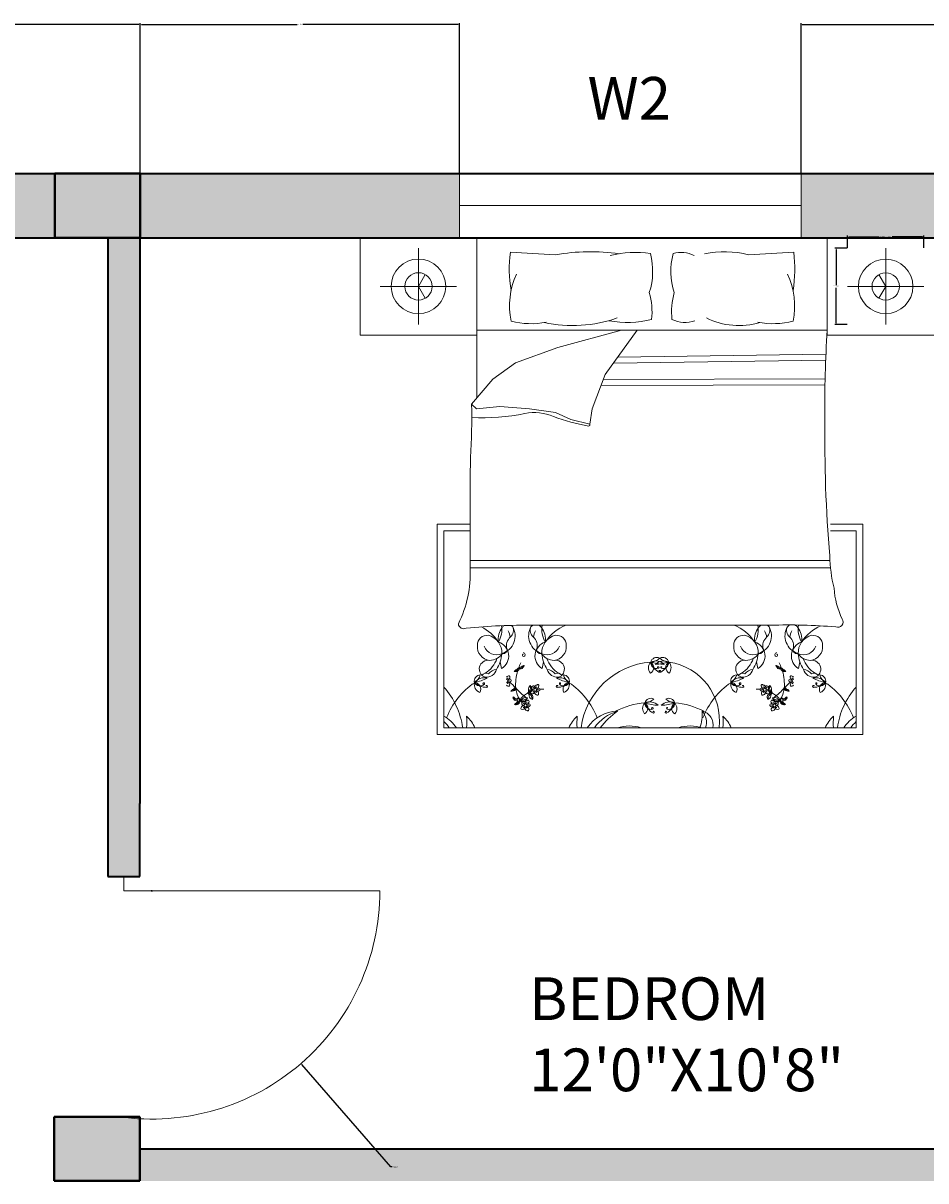
# Model space of a CAD drawing. Units: inches. Extents: x 1623 to 2200, y 2019 to 3010.
# Tile 4 of 6: x 1902 to 2029, y 2342 to 2505. Entities that reach past the tile are written whole.
import ezdxf

# ---------------------------------------------------------------- set-up
doc = ezdxf.new("R2010")
doc.units = ezdxf.units.IN
for name, color, linetype, lineweight in [('A-ANNO-DIMS', 2, 'Continuous', 18), ('A-AREA-IDEN', 7, 'Continuous', 18), ('A-COLS', 7, 'Continuous', 40), ('A-DOOR', 3, 'Continuous', 18), ('A-FURN', 8, 'Continuous', 13), ('A-GLAZ', 4, 'Continuous', 18), ('A-GLAZ-IDEN', 7, 'Continuous', 18), ('A-WALL', 7, 'Continuous', 35)]:
    doc.layers.add(name, color=color, linetype=linetype, lineweight=lineweight)
doc.layers.add('A-COLS-PATT', color=152, linetype='Continuous', lineweight=13, true_color=0x2776bb)
doc.layers.add('A-WALL-PATT', color=251, linetype='Continuous', lineweight=13, true_color=0x636466)
doc.styles.get("Standard").update_dxf_attribs({"font": 'arial.ttf'})
doc.dimstyles.get("Standard").update_dxf_attribs({"dimtxt": 0.18, "dimasz": 0.18, "dimexe": 0.18, "dimexo": 0.0625, "dimgap": 0.09, "dimtad": 0, "dimtih": 1, "dimtoh": 1, "dimdec": 4, "dimzin": 0, "dimdsep": 46, "dimtxsty": 'Standard', "dimcen": 0.09, "dimadec": 0, "dimazin": 0, "dimtfac": 1, "dimtdec": 4, "dimtofl": 0, "dimtmove": 0, "dimatfit": 3, "dimfxl": 1, "dimtolj": 1, "dimtzin": 0, "dimarcsym": 0})

# ---------------------------------------------------------------- blocks, each defined once
blk = doc.blocks.new('COL-12X9-PLAN')
for p, q in [((0, 0), (0, 9)), ((0, 9), (12, 9)), ((12, 9), (12, 0)), ((9, 0), (0, 0)), ((12, 0), (9, 0))]:
    blk.add_line(p, q)
blk = doc.blocks.new('WIN-48-PLAN')
for p, q in [((0, 9), (0, 0)), ((48, 4.5), (48, 9)), ((48, 9), (48, 0)), ((0, 0), (0, 4.5)), ((0, 4.5), (48, 4.5))]:
    blk.add_line(p, q)
blk = doc.blocks.new('BEDSIDE-LAMP-PLAN')
for p, q in [((5.36, 0), (5.36, 10.73)), ((0, 5.36), (10.73, 5.36))]:
    blk.add_line(p, q)
for points in [[(5.36, 5.36), (4.41, 7.02)], [(5.36, 5.36), (4.41, 3.7)]]:
    blk.add_lwpolyline(points)
for radius in [3.83, 1.92]:
    blk.add_circle((5.36, 5.36), radius)
blk = doc.blocks.new('*D16')
at = {"layer": 'A-ANNO-DIMS', "color": 0, "lineweight": -2, "transparency": 16777216}
for p, q in [((2017.8, 2473.11), (2017.8, 2474.84)), ((2017.98, 2474.66), (2022.26, 2474.66)), ((2028.34, 2474.66), (2024.06, 2474.66)), ((2028.52, 2473.11), (2028.52, 2474.84))]:
    blk.add_line(p, q, dxfattribs=at)
at = {"layer": 'A-ANNO-DIMS', "color": 0, "transparency": 16777216}
for points in [[(2017.98, 2474.69), (2017.98, 2474.63), (2017.8, 2474.66)], [(2028.34, 2474.69), (2028.34, 2474.63), (2028.52, 2474.66)]]:
    blk.add_solid(points, dxfattribs=at)
at = {"layer": 'Defpoints', "color": 0, "transparency": 16777216}
for p in [(2028.52, 2474.66), (2017.8, 2473.05), (2028.52, 2473.05)]:
    blk.add_point(p, dxfattribs=at)
at = {"layer": 'A-ANNO-DIMS', "color": 0, "transparency": 16777216, "insert": (2023.16, 2474.66), "char_height": 0.18, "attachment_point": 5}
blk.add_mtext('\\A1;LAMP 11 TYP.', dxfattribs=at)
blk = doc.blocks.new('*D17')
at = {"layer": 'A-ANNO-DIMS', "color": 0, "lineweight": -2, "transparency": 16777216}
for p, q in [((2017.73, 2473.05), (2016.01, 2473.05)), ((2016.19, 2472.87), (2016.19, 2467.86)), ((2016.19, 2462.5), (2016.19, 2467.5)), ((2017.73, 2462.32), (2016.01, 2462.32))]:
    blk.add_line(p, q, dxfattribs=at)
at = {"layer": 'A-ANNO-DIMS', "color": 0, "transparency": 16777216}
for points in [[(2016.16, 2472.87), (2016.22, 2472.87), (2016.19, 2473.05)], [(2016.16, 2462.5), (2016.22, 2462.5), (2016.19, 2462.32)]]:
    blk.add_solid(points, dxfattribs=at)
at = {"layer": 'Defpoints', "color": 0, "transparency": 16777216}
for p in [(2016.19, 2473.05), (2017.8, 2473.05), (2017.8, 2462.32)]:
    blk.add_point(p, dxfattribs=at)
at = {"layer": 'A-ANNO-DIMS', "color": 0, "transparency": 16777216, "insert": (2016.19, 2467.68), "char_height": 0.18, "attachment_point": 5}
blk.add_mtext('\\A1;11 TYP.', dxfattribs=at)
blk = doc.blocks.new('*D34')
at = {"layer": 'A-ANNO-DIMS', "color": 0, "lineweight": -2, "transparency": 16777216}
for p, q in [((1878.5, 2483.59), (1878.5, 2504.66)), ((1918.4, 2483.59), (1918.4, 2504.66)), ((1878.68, 2504.48), (1898.12, 2504.48)), ((1918.22, 2504.48), (1898.77, 2504.48))]:
    blk.add_line(p, q, dxfattribs=at)
at = {"layer": 'A-ANNO-DIMS', "color": 0, "transparency": 16777216}
for points in [[(1878.68, 2504.51), (1878.68, 2504.45), (1878.5, 2504.48)], [(1918.22, 2504.51), (1918.22, 2504.45), (1918.4, 2504.48)]]:
    blk.add_solid(points, dxfattribs=at)
at = {"layer": 'Defpoints', "color": 0, "transparency": 16777216}
for p in [(1918.4, 2504.48), (1878.5, 2483.52), (1918.4, 2483.52)]:
    blk.add_point(p, dxfattribs=at)
at = {"layer": 'A-ANNO-DIMS', "color": 0, "transparency": 16777216, "insert": (1898.45, 2504.48), "char_height": 0.18, "attachment_point": 5}
blk.add_mtext('\\A1;39.9', dxfattribs=at)
blk = doc.blocks.new('*D35')
at = {"layer": 'A-ANNO-DIMS', "color": 0, "lineweight": -2, "transparency": 16777216}
for p, q in [((1918.4, 2483.59), (1918.4, 2504.66)), ((1963.26, 2483.59), (1963.26, 2504.66)), ((1918.58, 2504.48), (1940.43, 2504.48)), ((1963.08, 2504.48), (1941.23, 2504.48))]:
    blk.add_line(p, q, dxfattribs=at)
at = {"layer": 'A-ANNO-DIMS', "color": 0, "transparency": 16777216}
for points in [[(1918.58, 2504.51), (1918.58, 2504.45), (1918.4, 2504.48)], [(1963.08, 2504.51), (1963.08, 2504.45), (1963.26, 2504.48)]]:
    blk.add_solid(points, dxfattribs=at)
at = {"layer": 'Defpoints', "color": 0, "transparency": 16777216}
for p in [(1963.26, 2504.48), (1918.4, 2483.52), (1963.26, 2483.52)]:
    blk.add_point(p, dxfattribs=at)
at = {"layer": 'A-ANNO-DIMS', "color": 0, "transparency": 16777216, "insert": (1940.83, 2504.48), "char_height": 0.18, "attachment_point": 5}
blk.add_mtext('\\A1;44.86', dxfattribs=at)
blk = doc.blocks.new('*D36')
at = {"layer": 'A-ANNO-DIMS', "color": 0, "lineweight": -2, "transparency": 16777216}
for p, q in [((2011.26, 2483.59), (2011.26, 2504.66)), ((2071.33, 2483.59), (2071.33, 2504.66)), ((2011.44, 2504.48), (2040.9, 2504.48)), ((2071.15, 2504.48), (2041.69, 2504.48))]:
    blk.add_line(p, q, dxfattribs=at)
at = {"layer": 'A-ANNO-DIMS', "color": 0, "transparency": 16777216}
for points in [[(2011.44, 2504.51), (2011.44, 2504.45), (2011.26, 2504.48)], [(2071.15, 2504.51), (2071.15, 2504.45), (2071.33, 2504.48)]]:
    blk.add_solid(points, dxfattribs=at)
at = {"layer": 'Defpoints', "color": 0, "transparency": 16777216}
for p in [(2071.33, 2504.48), (2011.26, 2483.52), (2071.33, 2483.53)]:
    blk.add_point(p, dxfattribs=at)
at = {"layer": 'A-ANNO-DIMS', "color": 0, "transparency": 16777216, "insert": (2041.29, 2504.48), "char_height": 0.18, "attachment_point": 5}
blk.add_mtext('\\A1;60.07', dxfattribs=at)
blk = doc.blocks.new('*D63')
at = {"layer": 'A-ANNO-DIMS', "color": 0, "lineweight": -2, "transparency": 16777216}
for p, q in [((1919.92, 2382.76), (1920.1, 2382.76)), ((1920.01, 2382.67), (1920.01, 2382.85)), ((1953.6, 2343.98), (1941.12, 2358.39)), ((1953.78, 2343.98), (1953.6, 2343.98))]:
    blk.add_line(p, q, dxfattribs=at)
at = {"layer": 'A-ANNO-DIMS', "color": 0, "transparency": 16777216}
blk.add_solid([(1941.15, 2358.41), (1941.1, 2358.37), (1941.01, 2358.53)], dxfattribs=at)
at = {"layer": 'Defpoints', "color": 0, "transparency": 16777216}
for p in [(1920.01, 2382.76), (1941.01, 2358.53)]:
    blk.add_point(p, dxfattribs=at)
at = {"layer": 'A-ANNO-DIMS', "color": 0, "transparency": 16777216, "insert": (1954.26, 2343.98), "char_height": 0.18, "attachment_point": 5}
blk.add_mtext('\\A1;R32.06', dxfattribs=at)

msp = doc.modelspace()

# ---------------------------------------------------------------- hatches: boundary and pattern name
at = {"layer": 'A-COLS-PATT'}
h = msp.add_hatch(color=256, dxfattribs=at)
h.dxf.hatch_style = 1
h.paths.add_polyline_path([(1722.3258, 2483.5237), (1710.3258, 2483.5237), (1710.3258, 2474.5237), (1719.3258, 2474.5237), (1722.3258, 2474.5237)])
h.paths.add_polyline_path([(1809.3258, 2483.5237), (1797.3258, 2483.5237), (1797.3258, 2474.5237), (1806.3258, 2474.5237), (1809.3258, 2474.5237)])
h.paths.add_polyline_path([(1918.3972, 2483.5237), (1906.3972, 2483.5237), (1906.3972, 2474.5237), (1915.3972, 2474.5237), (1918.3972, 2474.5237)])
h.paths.add_polyline_path([(2071.3258, 2483.5237), (2059.3258, 2483.5237), (2059.3258, 2474.532), (2068.3258, 2474.532), (2071.3258, 2474.532)])
h.paths.add_polyline_path([(2071.3258, 2351.0312), (2059.3258, 2351.0312), (2059.3258, 2342.0312), (2068.3258, 2342.0312), (2071.3258, 2342.0312)])
h.paths.add_polyline_path([(1918.3258, 2351.0237), (1906.3258, 2351.0237), (1906.3258, 2342.0237), (1915.3258, 2342.0237), (1918.3258, 2342.0237)])
h.paths.add_polyline_path([(1722.3198, 2351.0237), (1710.3258, 2351.0237), (1710.3258, 2342.0237), (1719.3198, 2342.0237), (1722.3198, 2342.0237)])
h.paths.add_polyline_path([(1809.3158, 2351.0237), (1797.3258, 2351.0237), (1797.3258, 2346.5237), (1797.3158, 2342.0237), (1806.3158, 2342.0237), (1809.3158, 2342.0237)])
h.paths.add_polyline_path([(1722.3029, 2170.0237), (1710.3258, 2170.0237), (1710.3258, 2161.0237), (1714.3029, 2161.0237), (1719.3029, 2161.0237), (1722.3029, 2161.0237)])
h.paths.add_polyline_path([(1809.3258, 2170.0237), (1797.3258, 2170.0237), (1797.3258, 2161.0237), (1801.3258, 2161.0237), (1802.9141, 2161.0237), (1806.3258, 2161.0237), (1809.3258, 2161.0237)])
h.paths.add_polyline_path([(1918.2273, 2170.0237), (1906.2273, 2170.0237), (1906.2273, 2161.0237), (1915.2273, 2161.0237), (1918.2273, 2161.0237)])
h.paths.add_polyline_path([(2071.3258, 2170.0237), (2059.3258, 2170.0237), (2059.3258, 2161.0237), (2068.3258, 2161.0237), (2071.3258, 2161.0237)])
at = {"layer": 'A-WALL-PATT'}
h = msp.add_hatch(color=256, dxfattribs=at)
h.dxf.hatch_style = 1
h.paths.add_polyline_path([(1725.9857, 2483.5237), (1722.3258, 2483.5237), (1722.3258, 2474.5237), (1725.9857, 2474.5237), (1725.9857, 2479.0237)])
h.paths.add_polyline_path([(1797.3258, 2483.5237), (1749.9857, 2483.5237), (1749.9857, 2474.5237), (1797.3258, 2474.5237)])
h.paths.add_polyline_path([(1830.4977, 2483.5237), (1809.3258, 2483.5237), (1809.3258, 2474.5237), (1830.4977, 2474.5237), (1830.4977, 2479.0237)])
h.paths.add_polyline_path([(1906.3972, 2483.5237), (1878.4977, 2483.5237), (1878.4977, 2474.5237), (1906.3972, 2474.5237)])
h.paths.add_polyline_path([(1918.3258, 2474.5237), (1915.3972, 2474.5237), (1913.8258, 2474.5237), (1913.8258, 2395.0237), (1913.8258, 2384.7587), (1918.3258, 2384.7587), (1918.3258, 2395.0237)])
h.paths.add_polyline_path([(1801.8258, 2474.5237), (1797.3258, 2474.5237), (1797.3258, 2436.0951), (1801.8258, 2436.0951)], flags=17)
h.paths.add_polyline_path([(1719.3258, 2474.5237), (1710.3258, 2474.5237), (1710.3258, 2351.0237), (1719.3258, 2351.0237), (1719.3258, 2395.0237), (1801.8258, 2395.0237), (1801.8258, 2399.5237), (1719.3258, 2399.5237)])
h.paths.add_polyline_path([(1797.3158, 2346.5237), (1722.3198, 2346.5237), (1722.3198, 2342.0237), (1797.3158, 2342.0237)])
h.paths.add_polyline_path([(1801.8258, 2361.4421), (1797.3258, 2361.4421), (1797.3258, 2351.0237), (1801.8258, 2351.0237)], flags=17)
h.paths.add_polyline_path([(2059.3258, 2346.5237), (1918.3258, 2346.5237), (1918.3258, 2342.0237), (2059.3258, 2342.0237)])
h.paths.add_polyline_path([(1963.26, 2479.0237), (1963.26, 2483.5237), (1918.3972, 2483.5237), (1918.3972, 2474.5237), (1963.26, 2474.5237)])
h.paths.add_polyline_path([(2059.3258, 2483.5237), (2011.26, 2483.5237), (2011.26, 2474.5237), (2059.3258, 2474.5237)])
h.paths.add_polyline_path([(2071.3258, 2474.532), (2068.3258, 2474.532), (2062.3258, 2474.532), (2062.3258, 2351.0312), (2071.3258, 2351.0312)])
h.paths.add_polyline_path([(2071.3258, 2342.0312), (2068.3258, 2342.0312), (2062.3258, 2342.0312), (2062.3258, 2170.0237), (2071.3258, 2170.0237)])
h.paths.add_polyline_path([(2059.3258, 2170.0237), (2038.3258, 2170.0237), (2038.3258, 2161.0237), (2059.3258, 2161.0237)])
h.paths.add_polyline_path([(1990.3258, 2170.0237), (1963.4402, 2170.0237), (1963.4402, 2161.0237), (1990.3258, 2161.0237), (1990.3258, 2165.5237)])
h.paths.add_polyline_path([(1918.3258, 2274.595), (1913.8258, 2274.595), (1913.8258, 2170.0237), (1918.3258, 2170.0237)])
h.paths.add_polyline_path([(1906.2273, 2170.0237), (1871.454, 2170.0237), (1871.454, 2161.0237), (1906.2273, 2161.0237)])
h.paths.add_polyline_path([(1835.454, 2170.0237), (1809.3258, 2170.0237), (1809.3258, 2161.0237), (1835.454, 2161.0237), (1835.454, 2165.5237)])
h.paths.add_polyline_path([(1801.8258, 2270.095), (1865.2406, 2270.095), (1865.2406, 2274.595), (1797.3258, 2274.595), (1797.3258, 2170.0237), (1801.8258, 2170.0237)])
h.paths.add_polyline_path([(1719.3258, 2342.0237), (1719.3198, 2342.0237), (1710.3258, 2342.0237), (1710.3258, 2170.0237), (1719.3258, 2170.0237)])

# ---------------------------------------------------------------- linework, layer by layer
at = {"layer": 'A-DOOR'}
for p, q in [((1916.0758, 2384.7587), (1916.0758, 2382.7587)), ((1916.0758, 2382.7587), (1952.0758, 2382.7587))]:
    msp.add_line(p, q, dxfattribs=at)
msp.add_arc((1920.0132, 2382.7587), 32.0625, 261.802931, 0, dxfattribs=at)
at = {"layer": 'A-FURN'}
for p, q in [((2031.3673, 2474.5237), (1949.2842, 2474.5237)), ((1965.7008, 2474.5237), (1965.7008, 2451.9942)), ((1965.7008, 2461.5522), (2014.9507, 2461.5522)), ((1977.1025, 2459.1126), (1986.0533, 2461.5522)), ((1988.2506, 2461.5522), (1983.7526, 2455.2911)), ((1971.1173, 2456.9526), (1977.1025, 2459.1126)), ((2014.7304, 2458.1421), (1985.5065, 2457.7325)), ((1967.9585, 2454.6265), (1971.1173, 2456.9526)), ((2014.6985, 2457.2997), (1984.8933, 2456.8789)), ((1964.9659, 2451.1374), (1967.9585, 2454.6265)), ((1983.7526, 2455.2911), (1981.9239, 2450.4728)), ((2014.6561, 2454.7154), (1983.4871, 2454.5915)), ((2014.6604, 2453.8726), (1983.1652, 2453.7435)), ((1965.631, 2450.4728), (1964.9659, 2451.1374)), ((1968.956, 2450.8051), (1965.631, 2450.4728)), ((1973.1124, 2450.4728), (1968.956, 2450.8051)), ((1976.77, 2449.9744), (1973.1124, 2450.4728)), ((1978.9313, 2448.9775), (1976.77, 2449.9744)), ((1981.9239, 2450.4728), (1981.5913, 2448.3129)), ((1981.5913, 2448.3129), (1978.9313, 2448.9775)), ((1960.1184, 2434.2863), (1964.7614, 2434.2863)), ((1960.1184, 2404.7176), (1960.1184, 2434.2863)), ((1964.7596, 2433.3351), (1961.0696, 2433.3351)), ((1961.0696, 2433.3351), (1961.0696, 2405.6688)), ((2019.0092, 2433.3351), (2015.391, 2433.3351)), ((2015.4083, 2434.2863), (2019.9604, 2434.2863)), ((2019.0092, 2405.6688), (2019.0092, 2433.3351)), ((2019.9604, 2434.2863), (2019.9604, 2404.7176)), ((2015.3236, 2429.1669), (1964.7551, 2429.1669)), ((2015.4016, 2428.1431), (1964.7549, 2428.1431)), ((2006.9893, 2420.0802), (1973.6623, 2420.0802)), ((1969.1584, 2413.9906), (1968.9769, 2414.9181)), ((1974.8951, 2413.9906), (1975.0766, 2414.9181)), ((2005.1837, 2413.9906), (2005.0022, 2414.9181)), ((2010.9204, 2413.9906), (2011.1018, 2414.9181)), ((1961.0696, 2405.6688), (2019.0092, 2405.6688)), ((2019.9604, 2404.7176), (1960.1184, 2404.7176))]:
    msp.add_line(p, q, dxfattribs=at)
for points in [[(1965.7008, 2460.8432), (1949.2842, 2460.8432), (1949.2842, 2474.5237)], [(2014.9507, 2474.5237), (2014.9507, 2460.8432), (2031.3673, 2460.8432), (2031.3673, 2474.5237)]]:
    msp.add_lwpolyline(points, dxfattribs=at)
for points in [[(1970.4154, 2472.4779, 0.07489676), (1970.515, 2467.1165, -0.47281659)], [(1989.9412, 2466.8166, 0.14098958), (1990.1054, 2472.2862, 0.23524475)], [(1993.4464, 2466.8166, -0.14098958), (1993.2822, 2472.2862, -0.23524475)], [(2010.2361, 2472.4779, -0.07489676), (2010.1365, 2467.1165, 0.47281659)], [(1964.7942, 2443.6214, 0.00124232), (1964.7549, 2428.0471, -0.12720156), (1963.1094, 2420.2852)], [(2015.3011, 2429.8131, 0.05611182), (2015.8966, 2425.297, 0.09534134), (2017.0503, 2420.947)]]:
    msp.add_lwpolyline(points, format="xyb", dxfattribs=at)
for centre in [(1973.9006, 2411.0162), (2006.1782, 2411.0162), (1972.5333, 2408.8128), (2007.5455, 2408.8128)]:
    msp.add_circle(centre, 0.209, dxfattribs=at)
for centre, radius, start, end in [((2015.6592, 3253.6379), 782.4691, 266.6852093, 267.1497753), ((1981.6625, 2442.7753), 29.7695, 82.219583, 99.496983), ((1987.9498, 2457.8197), 14.6262, 81.524927, 103.959959), ((1994.4085, 2468.3849), 4.0606, 63.343742, 106.102557), ((2000.4939, 2458.1152), 14.4296, 76.342714, 101.1841), ((1964.9924, 3253.6379), 782.4691, 272.8502247, 273.3147907), ((1980.873, 2464.964), 10.5793, 155.1316, 191.758341), ((1999.7786, 2464.964), 10.5793, 348.241659, 24.8684), ((1980.2652, 2464.0732), 10.0574, 354.012888, 15.829277), ((2003.1225, 2464.0732), 10.0574, 164.170723, 185.987112), ((1973.3435, 2473.4386), 11.0002, 255.103933, 281.036887), ((1979.1342, 2481.2575), 19.0789, 258.039745, 289.261524), ((1986.8582, 2477.0919), 14.4751, 259.861689, 283.623756), ((1994.9576, 2466.9685), 4.3514, 245.01826, 288.540728), ((2002.5605, 2472.628), 10.4488, 243.876108, 286.174639), ((2007.3081, 2473.4386), 11.0002, 258.963113, 284.896067), ((2162.0989, 2451.5205), 147.4898, 176.099968, 180.928176), ((1889.7043, 2449.0969), 75.2893, 355.829411, 1.553045), ((1966.3707, 2480.2049), 30.9793, 267.45188, 281.339199), ((1973.7755, 2443.2791), 6.6817, 66.261584, 101.339199), ((1987.2903, 2479.331), 31.8326, 250.119422, 259.33829), ((1981.4049, 2448.2459), 0.1981, 268.862345, 19.753635), ((2206.9989, 2446.1582), 192.3933, 179.114536, 184.873507), ((1963.8649, 2420.3378), 0.7574, 183.979981, 297.341241), ((1972.6828, 2334.6364), 85.4494, 89.343254, 95.688691), ((1974.0179, 2419.1722), 0.9886, 113.229008, 135.548308), ((1974.0179, 2419.1722), 0.9886, 37.675028, 66.714357), ((1978.23, 2419.4729), 3.4007, 169.713345, 211.178216), ((1980.5086, 2414.2998), 6.2125, 111.494132, 146.332878), ((1999.5702, 2414.2998), 6.2125, 33.667122, 68.505868), ((2001.8487, 2419.4729), 3.4007, 328.821784, 10.286655), ((2006.0609, 2419.1722), 0.9886, 113.285643, 142.324972), ((2006.0609, 2419.1722), 0.9886, 44.451692, 66.714357), ((2009.503, 2340.2466), 79.8732, 85.240242, 91.803508), ((2010.0432, 2419.1722), 0.9886, 106.634335, 135.548308), ((2010.0432, 2419.1722), 0.9886, 37.675028, 72.581425), ((2014.2553, 2419.4729), 3.4007, 169.248989, 211.178216), ((2016.4288, 2420.5305), 0.7482, 246.521858, 33.826416), ((1967.1639, 2417.2828), 1.3859, 84.485571, 181.05378), ((1963.5449, 2414.2998), 6.2125, 33.667122, 63.299656), ((1966.7384, 2416.2575), 2.4688, 355.293344, 76.920995), ((1971.8709, 2417.9963), 3.1656, 145.785047, 184.730373), ((1965.8234, 2419.4729), 3.4007, 328.821784, 9.155424), ((1970.0356, 2419.1722), 0.9886, 120.029301, 142.324972), ((1968.4573, 2418.5893), 2.6158, 289.282177, 29.1751), ((1971.5491, 2417.1901), 1.6828, 131.565306, 195.147127), ((1968.0624, 2418.116), 2.3595, 7.435988, 29.914865), ((1969.6178, 2419.3681), 1.2282, 311.565306, 23.835407), ((1970.0356, 2419.1722), 0.9886, 44.451692, 63.558008), ((1975.5962, 2418.5893), 2.6158, 150.8249, 250.717823), ((1974.4357, 2419.3681), 1.2282, 156.164593, 228.434694), ((1972.5043, 2417.1901), 1.6828, 344.852873, 48.434694), ((1975.9911, 2418.116), 2.3595, 150.085135, 172.564012), ((1972.1826, 2417.9963), 3.1656, 355.269627, 34.214953), ((1977.3151, 2416.2575), 2.4688, 103.079005, 184.706656), ((1976.8896, 2417.2828), 1.3859, 358.94622, 95.514429), ((2003.1892, 2417.2828), 1.3859, 84.485571, 181.05378), ((2002.7637, 2416.2575), 2.4688, 355.293344, 76.920995), ((2007.8962, 2417.9963), 3.1656, 145.785047, 184.730373), ((2004.4826, 2418.5893), 2.6158, 289.282177, 29.1751), ((2007.5744, 2417.1901), 1.6828, 131.565306, 195.147127), ((2004.0877, 2418.116), 2.3595, 7.435988, 29.914865), ((2005.643, 2419.3681), 1.2282, 311.565306, 23.835407), ((2011.6215, 2418.5893), 2.6158, 150.8249, 250.717823), ((2010.461, 2419.3681), 1.2282, 156.164593, 228.434694), ((2008.5296, 2417.1901), 1.6828, 344.852873, 48.434694), ((2012.0164, 2418.116), 2.3595, 150.085135, 172.564012), ((2008.2079, 2417.9963), 3.1656, 355.269627, 34.214953), ((2013.3404, 2416.2575), 2.4688, 103.079005, 184.706656), ((2016.5339, 2414.2998), 6.2125, 113.645326, 146.332878), ((2012.9149, 2417.2828), 1.3859, 358.94622, 95.514429), ((1967.7322, 2417.0845), 1.9615, 174.944852, 262.885747), ((1968.5031, 2417.8282), 1.9049, 201.581867, 291.422148), ((1968.1409, 2415.7595), 2.0406, 299.908541, 73.133701), ((1975.9126, 2415.7595), 2.0406, 106.866299, 240.091459), ((1975.5503, 2417.8282), 1.9049, 248.577852, 338.418133), ((1976.3213, 2417.0845), 1.9615, 277.114253, 5.055148), ((2003.7575, 2417.0845), 1.9615, 174.944852, 262.885747), ((2004.5284, 2417.8282), 1.9049, 201.581867, 291.422148), ((2004.1662, 2415.7595), 2.0406, 299.908541, 73.133701), ((2011.9379, 2415.7595), 2.0406, 106.866299, 240.091459), ((2011.5756, 2417.8282), 1.9049, 248.577852, 338.418133), ((2012.3466, 2417.0845), 1.9615, 277.114253, 5.055148), ((1964.8385, 2416.6355), 3.8752, 301.261374, 341.704505), ((1967.3911, 2417.5204), 2.3844, 272.359103, 324.040141), ((1964.8022, 2416.3232), 4.4049, 326.288284, 356.507596), ((1971.8709, 2417.9963), 3.1656, 212.70113, 216.34448), ((1969.4331, 2416.6172), 0.5095, 257.304058, 15.147127), ((1972.2623, 2415.8444), 0.1582, 102.70507, 280.438449), ((1972.2444, 2415.9418), 0.2572, 280.438449, 100.413559), ((1974.6204, 2416.6172), 0.5095, 164.852873, 282.695942), ((1972.1826, 2417.9963), 3.1656, 323.65552, 327.29887), ((1976.6624, 2417.5204), 2.3844, 215.959859, 267.640897), ((1979.2513, 2416.3232), 4.4049, 183.492404, 213.711716), ((1979.215, 2416.6355), 3.8752, 198.295495, 238.738626), ((1990.9833, 2414.6628), 0.8886, 63.027371, 163.803749), ((1990.0833, 2416.7408), 1.8308, 271.458456, 315.372663), ((1991.8316, 2414.6628), 0.8886, 16.196251, 116.972629), ((1992.7315, 2416.7408), 1.8308, 224.627337, 268.541544), ((2000.8638, 2416.6355), 3.8752, 301.261374, 341.704505), ((2003.4164, 2417.5204), 2.3844, 272.359103, 324.040141), ((2000.8275, 2416.3232), 4.4049, 326.288284, 356.507596), ((2007.8962, 2417.9963), 3.1656, 212.70113, 216.34448), ((2005.4583, 2416.6172), 0.5095, 257.304058, 15.147127), ((2007.8344, 2415.9418), 0.2572, 79.586441, 259.561551), ((2007.8164, 2415.8444), 0.1582, 259.561551, 77.29493), ((2010.6457, 2416.6172), 0.5095, 164.852873, 282.695942), ((2008.2079, 2417.9963), 3.1656, 323.65552, 327.29887), ((2012.6877, 2417.5204), 2.3844, 215.959859, 267.640897), ((2015.2766, 2416.3232), 4.4049, 183.492404, 213.711716), ((2015.2403, 2416.6355), 3.8752, 198.295495, 238.738626), ((1967.2809, 2413.9239), 1.2319, 80.263976, 250.868843), ((1966.9854, 2414.2946), 1.5383, 265.969018, 344.304497), ((1968.6423, 2412.2496), 1.6384, 96.166203, 141.582546), ((1971.3558, 2413.3991), 0.431, 101.325614, 154.46214), ((1970.7359, 2414.8615), 1.2973, 280.258782, 300.655993), ((1971.0346, 2415.8987), 2.3149, 268.326386, 277.130238), ((1977.9519, 2411.7129), 6.7985, 163.584179, 183.827683), ((1970.4555, 2414.8579), 1.3188, 308.210121, 316.307119), ((1971.2648, 2413.9915), 0.3939, 278.343222, 4.286854), ((1971.0467, 2414.3372), 0.6879, 300.655993, 332.634143), ((1971.5635, 2413.8827), 0.1673, 55.765747, 157.441651), ((1977.9519, 2411.7129), 6.7985, 153.003195, 159.894078), ((1971.8239, 2414.0386), 0.1673, 84.378377, 186.054275), ((1971.6674, 2414.7088), 0.6879, 269.185879, 301.164033), ((1971.8691, 2414.3534), 0.3939, 237.533168, 323.476805), ((1971.4876, 2415.4758), 1.3188, 285.512908, 293.609906), ((1972.3483, 2413.9933), 0.431, 87.357882, 140.494412), ((1971.352, 2415.2303), 1.2973, 301.164033, 321.561245), ((1970.2966, 2415.4569), 2.3149, 324.689789, 333.493639), ((1975.4112, 2412.2496), 1.6384, 38.417454, 83.833797), ((1977.0681, 2414.2946), 1.5383, 195.695503, 274.030982), ((1976.7725, 2413.9239), 1.2319, 289.131157, 99.736024), ((1990.9639, 2404.2242), 10.7189, 94.462329, 172.255043), ((1991.0103, 2414.112), 1.1887, 137.787318, 219.114465), ((1989.6604, 2414.1485), 0.8952, 298.539099, 58.362682), ((1991.0061, 2414.8763), 0.8769, 177.758486, 283.85198), ((1990.8276, 2413.3663), 1.6946, 45.541131, 114.310082), ((1992.3732, 2422.0658), 7.4986, 252.593037, 267.258174), ((1992.6944, 2415.7894), 2.7108, 198.915948, 238.010978), ((1991.9873, 2413.3663), 1.6946, 65.689918, 134.458869), ((1990.4417, 2422.0658), 7.4986, 272.741826, 287.406963), ((1991.1883, 2414.1376), 0.116, 283.85198, 219.924541), ((1991.3288, 2413.6032), 0.1331, 238.010978, 71.559179), ((1991.3505, 2413.6681), 0.0647, 71.559179, 188.016679), ((1991.486, 2413.6032), 0.1331, 108.440821, 301.989022), ((1991.4644, 2413.6681), 0.0647, 351.983321, 108.440821), ((1991.6155, 2414.1823), 0.0699, 320.190924, 256.020882), ((1990.1205, 2415.7894), 2.7108, 301.989022, 341.084052), ((1991.8087, 2414.8763), 0.8769, 256.14802, 2.241514), ((1993.1545, 2414.1485), 0.8952, 121.637318, 241.460901), ((1991.8045, 2414.112), 1.1887, 320.885535, 42.212682), ((1991.5045, 2406.6994), 8.2957, 352.863554, 81.819659), ((2003.3062, 2413.9239), 1.2319, 80.263976, 250.868843), ((2003.0106, 2414.2946), 1.5383, 265.969018, 344.304497), ((2004.6676, 2412.2496), 1.6384, 96.166203, 141.582546), ((2007.7305, 2413.9933), 0.431, 39.505588, 92.642118), ((2008.7268, 2415.2303), 1.2973, 218.438755, 238.835967), ((2009.7821, 2415.4569), 2.3149, 206.506361, 215.310211), ((2008.2097, 2414.3534), 0.3939, 216.523195, 302.466832), ((2008.4114, 2414.7088), 0.6879, 238.835967, 270.814121), ((2008.5912, 2415.4758), 1.3188, 246.390094, 254.487092), ((2002.1269, 2411.7129), 6.7985, 20.105922, 26.996805), ((2008.2548, 2414.0386), 0.1673, 353.945725, 95.621623), ((2008.814, 2413.9915), 0.3939, 175.713146, 261.656778), ((2008.5153, 2413.8827), 0.1673, 22.558349, 124.234253), ((2009.0321, 2414.3372), 0.6879, 207.365857, 239.344007), ((2002.1269, 2411.7129), 6.7985, 356.172317, 16.415821), ((2009.6233, 2414.8579), 1.3188, 223.692881, 231.789879), ((2009.3428, 2414.8615), 1.2973, 239.344007, 259.741218), ((2009.0442, 2415.8987), 2.3149, 262.869762, 271.673614), ((2008.7229, 2413.3991), 0.431, 25.53786, 78.674386), ((2013.0934, 2414.2946), 1.5383, 195.695503, 274.030982), ((2011.4365, 2412.2496), 1.6384, 38.417454, 83.833797), ((2012.7978, 2413.9239), 1.2319, 289.131157, 99.736024), ((1971.4279, 2403.1645), 10.7189, 124.386545, 158.590793), ((1966.5356, 2411.7572), 1.1887, 167.711531, 249.038678), ((1966.2374, 2412.2211), 0.8886, 92.951587, 193.727964), ((1964.4208, 2413.5731), 1.8308, 301.382672, 345.296877), ((1966.7492, 2411.0197), 1.6946, 75.465349, 144.234293), ((1963.749, 2419.3305), 7.4986, 282.517257, 297.18239), ((1965.3474, 2411.1154), 0.8952, 328.463314, 88.286895), ((1967.1583, 2414.0511), 2.7108, 228.840165, 267.935195), ((1966.1506, 2412.4175), 0.8769, 207.682699, 313.776193), ((1967.0273, 2412.5891), 0.755, 63.975548, 143.268054), ((1966.6771, 2411.8681), 0.116, 313.776193, 249.718346), ((1970.1372, 2412.5823), 0.3487, 101.563728, 142.635797), ((1969.8481, 2412.2585), 0.209, 273.276835, 86.723165), ((1970.0918, 2412.4563), 0.1996, 91.108054, 181.867469), ((1970.5055, 2412.3312), 0.6347, 203.427571, 227.610371), ((1970.3038, 2412.0547), 0.4321, 80.348696, 133.653825), ((1970.2264, 2412.4122), 0.3421, 229.788918, 317.679152), ((1969.8573, 2412.8555), 0.5027, 288.726271, 352.503155), ((1969.8408, 2411.6879), 0.4858, 355.053037, 68.361764), ((1970.2218, 2411.6056), 0.6843, 83.085162, 105.717093), ((1970.1995, 2412.8311), 0.1615, 345.235561, 144.924803), ((1965.483, 2405.9285), 7.7936, 43.154125, 52.045905), ((1970.3461, 2412.3032), 0.1801, 317.679152, 80.348696), ((1977.0261, 2412.5891), 0.755, 36.731946, 116.024452), ((1977.3043, 2411.0197), 1.6946, 35.765707, 104.534651), ((1980.3045, 2419.3305), 7.4986, 242.81761, 257.482743), ((1976.8951, 2414.0511), 2.7108, 272.064805, 311.159835), ((1977.9028, 2412.4175), 0.8769, 226.223807, 332.317301), ((1977.3892, 2411.9124), 0.0699, 290.266709, 226.227077), ((1978.7061, 2411.1154), 0.8952, 91.713105, 211.536686), ((1977.8161, 2412.2211), 0.8886, 346.272036, 87.048413), ((1979.6327, 2413.5731), 1.8308, 194.703123, 238.617328), ((1977.5179, 2411.7572), 1.1887, 290.961322, 12.288469), ((1972.6256, 2403.1645), 10.7189, 21.409207, 55.613455), ((2007.4532, 2403.1645), 10.7189, 124.386545, 158.590793), ((2002.5609, 2411.7572), 1.1887, 167.711531, 249.038678), ((2002.2627, 2412.2211), 0.8886, 92.951587, 193.727964), ((2000.446, 2413.5731), 1.8308, 301.382672, 345.296877), ((2002.7745, 2411.0197), 1.6946, 75.465349, 144.234293), ((1999.7742, 2419.3305), 7.4986, 282.517257, 297.18239), ((2002.1759, 2412.4175), 0.8769, 207.682699, 313.776193), ((2003.1836, 2414.0511), 2.7108, 228.840165, 267.935195), ((2001.3727, 2411.1154), 0.8952, 328.463314, 88.286895), ((2003.0526, 2412.5891), 0.755, 63.975548, 143.268054), ((2002.7024, 2411.8681), 0.116, 313.776193, 249.718346), ((2014.5958, 2405.9285), 7.7936, 127.954095, 136.845875), ((2009.7327, 2412.3032), 0.1801, 99.651304, 222.320848), ((2009.8524, 2412.4122), 0.3421, 222.320848, 310.211082), ((2009.7749, 2412.0547), 0.4321, 46.346175, 99.651304), ((2009.8793, 2412.8311), 0.1615, 35.075197, 194.764439), ((2010.2215, 2412.8555), 0.5027, 187.496845, 251.273729), ((2010.238, 2411.6879), 0.4858, 111.638236, 184.946963), ((2009.857, 2411.6056), 0.6843, 74.282907, 96.914838), ((2009.987, 2412.4563), 0.1996, 358.132531, 88.891946), ((2009.5733, 2412.3312), 0.6347, 312.389629, 336.572429), ((2009.9416, 2412.5823), 0.3487, 37.364203, 78.436272), ((2010.2306, 2412.2585), 0.209, 93.276835, 266.723165), ((2013.0514, 2412.5891), 0.755, 36.731946, 116.024452), ((2013.3296, 2411.0197), 1.6946, 35.765707, 104.534651), ((2016.3298, 2419.3305), 7.4986, 242.81761, 257.482743), ((2012.9204, 2414.0511), 2.7108, 272.064805, 311.159835), ((2013.9281, 2412.4175), 0.8769, 226.223807, 332.317301), ((2013.4144, 2411.9124), 0.0699, 290.266709, 226.227077), ((2014.7314, 2411.1154), 0.8952, 91.713105, 211.536686), ((2015.658, 2413.5731), 1.8308, 194.703123, 238.617328), ((2013.8414, 2412.2211), 0.8886, 346.272036, 87.048413), ((2013.5432, 2411.7572), 1.1887, 290.961322, 12.288469), ((2008.6509, 2403.1645), 10.7189, 21.409207, 55.613455), ((1953.0896, 2404.2242), 10.7189, 7.744957, 41.885603), ((1967.0518, 2411.5422), 0.0647, 101.483395, 217.940894), ((1967.0655, 2411.4751), 0.1331, 267.935195, 101.483395), ((1970.1329, 2411.8714), 0.3451, 217.762086, 259.040263), ((1970.165, 2411.6598), 0.1604, 232.473712, 355.053037), ((1970.8668, 2410.6371), 0.431, 101.325614, 154.46214), ((1970.2469, 2412.0995), 1.2973, 280.258782, 300.655993), ((1970.5456, 2413.1368), 2.3149, 268.326386, 277.130238), ((1969.9664, 2412.0959), 1.3188, 308.210121, 316.307119), ((1970.7757, 2411.2296), 0.3939, 278.343222, 4.286854), ((1970.5576, 2411.5752), 0.6879, 300.655993, 332.634143), ((1971.0745, 2411.1208), 0.1673, 55.765747, 157.441651), ((1974.565, 2411.5416), 3.4082, 184.756021, 209.204084), ((1979.4716, 2418.7987), 11.2155, 222.241244, 232.174439), ((1974.9156, 2407.0148), 4.0882, 120.544017, 139.817977), ((1972.8091, 2411.1142), 0.5792, 272.849877, 356.122608), ((1972.3003, 2411.3269), 0.9528, 304.536861, 16.369906), ((1972.4001, 2410.889), 0.5608, 321.760733, 7.925193), ((1972.518, 2410.0832), 0.5608, 8.722715, 54.887172), ((1972.5478, 2409.6352), 0.9528, 0.278003, 72.111048), ((1973.6231, 2411.0593), 0.674, 127.310451, 187.925193), ((1972.9744, 2409.9847), 0.5792, 20.5253, 88.5375), ((1972.6973, 2411.1352), 0.6923, 355.010636, 41.65801), ((1973.4613, 2410.6239), 0.2071, 148.049899, 225.626809), ((1974.9156, 2407.0148), 4.0882, 113.050074, 113.847739), ((1973.8448, 2410.3847), 0.6591, 104.755814, 148.049899), ((1973.4749, 2410.8567), 0.4125, 247.408573, 351.438586), ((1973.6698, 2411.307), 0.2851, 126.104556, 271.428111), ((1973.6381, 2411.3844), 0.2048, 353.752558, 131.70535), ((1973.591, 2410.8399), 0.1385, 262.906013, 7.131983), ((1973.4454, 2411.141), 0.2877, 0.064508, 61.150746), ((1973.5138, 2411.3863), 0.3288, 311.84125, 355.787705), ((1974.1854, 2410.6291), 0.3451, 151.219585, 259.040263), ((1974.1896, 2411.34), 0.3487, 101.563728, 176.365034), ((1974.1442, 2411.214), 0.1996, 91.108054, 181.867469), ((1974.5579, 2411.0889), 0.6347, 203.427571, 227.610371), ((1974.3563, 2410.8124), 0.4321, 80.348696, 133.653825), ((1974.2788, 2411.1699), 0.3421, 229.788918, 317.679152), ((1973.9097, 2411.6132), 0.5027, 288.726271, 352.503155), ((1973.8932, 2410.4456), 0.4858, 355.053037, 68.361764), ((1974.2742, 2410.3633), 0.6843, 83.085162, 105.717093), ((1974.2519, 2411.5888), 0.1615, 345.235561, 144.924803), ((1974.2174, 2410.4175), 0.1604, 232.473712, 355.053037), ((1974.3985, 2411.0609), 0.1801, 317.679152, 80.348696), ((1974.9156, 2407.0148), 4.0882, 87.107093, 94.758526), ((1976.988, 2411.4751), 0.1331, 78.516605, 272.064805), ((1977.0017, 2411.5422), 0.0647, 322.059106, 78.516605), ((2003.0771, 2411.5422), 0.0647, 101.483395, 217.940894), ((2003.0907, 2411.4751), 0.1331, 267.935195, 101.483395), ((2005.1632, 2407.0148), 4.0882, 85.241474, 92.892907), ((2005.6803, 2411.0609), 0.1801, 99.651304, 222.320848), ((2005.8, 2411.1699), 0.3421, 222.320848, 310.211082), ((2005.7225, 2410.8124), 0.4321, 46.346175, 99.651304), ((2005.8268, 2411.5888), 0.1615, 35.075197, 194.764439), ((2006.169, 2411.6132), 0.5027, 187.496845, 251.273729), ((2006.1855, 2410.4456), 0.4858, 111.638236, 184.946963), ((2005.8613, 2410.4175), 0.1604, 184.946963, 307.526288), ((2005.8045, 2410.3633), 0.6843, 74.282907, 96.914838), ((2005.9346, 2411.214), 0.1996, 358.132531, 88.891946), ((2005.5208, 2411.0889), 0.6347, 312.389629, 336.572429), ((2005.8891, 2411.34), 0.3487, 3.634966, 78.436272), ((2005.8934, 2410.6291), 0.3451, 280.959737, 28.780415), ((2006.6038, 2410.8567), 0.4125, 188.561414, 292.591427), ((2006.4407, 2411.3844), 0.2048, 48.29465, 186.247442), ((2006.565, 2411.3863), 0.3288, 184.212295, 228.15875), ((2006.6334, 2411.141), 0.2877, 118.849254, 179.935492), ((2006.4877, 2410.8399), 0.1385, 172.868017, 277.093987), ((2006.409, 2411.307), 0.2851, 268.571889, 53.895444), ((2006.234, 2410.3847), 0.6591, 31.950101, 75.244186), ((2007.1044, 2409.9847), 0.5792, 91.4625, 159.4747), ((2007.5309, 2409.6352), 0.9528, 107.888952, 179.721997), ((2007.3815, 2411.1352), 0.6923, 138.34199, 184.989364), ((2007.2696, 2411.1142), 0.5792, 183.877392, 267.150123), ((2006.6175, 2410.6239), 0.2071, 314.373191, 31.950101), ((2005.1632, 2407.0148), 4.0882, 66.152261, 66.949926), ((2007.7784, 2411.3269), 0.9528, 163.630094, 235.463139), ((2006.4556, 2411.0593), 0.674, 352.074807, 52.689549), ((2007.5608, 2410.0832), 0.5608, 125.112828, 171.277285), ((2007.6787, 2410.889), 0.5608, 172.074807, 218.239267), ((2005.1632, 2407.0148), 4.0882, 40.182023, 59.455983), ((2000.6071, 2418.7987), 11.2155, 307.825561, 317.758756), ((2005.5137, 2411.5416), 3.4082, 330.795916, 355.243979), ((2009.303, 2411.2296), 0.3939, 175.713146, 261.656778), ((2009.0043, 2411.1208), 0.1673, 22.558349, 124.234253), ((2009.5211, 2411.5752), 0.6879, 207.365857, 239.344007), ((2010.1123, 2412.0959), 1.3188, 223.692881, 231.789879), ((2009.8319, 2412.0995), 1.2973, 239.344007, 259.741218), ((2009.5332, 2413.1368), 2.3149, 262.869762, 271.673614), ((2009.2119, 2410.6371), 0.431, 25.53786, 78.674386), ((2009.9138, 2411.6598), 0.1604, 184.946963, 307.526288), ((2009.9458, 2411.8714), 0.3451, 280.959737, 322.237914), ((2013.0133, 2411.4751), 0.1331, 78.516605, 272.064805), ((2013.0269, 2411.5422), 0.0647, 322.059106, 78.516605), ((2026.9892, 2404.2242), 10.7189, 138.114397, 172.255043), ((1971.0123, 2409.8812), 0.2334, 146.863595, 236.902126), ((1974.3032, 2415.0227), 6.107, 235.188198, 238.884407), ((1971.4125, 2410.2195), 0.6319, 199.479868, 267.68284), ((1971.3422, 2409.9806), 0.5442, 212.815476, 277.399174), ((1971.0257, 2409.6169), 0.6319, 266.970073, 338.291288), ((1967.695, 2414.1262), 6.107, 302.678403, 306.37461), ((1971.185, 2409.1176), 0.2334, 214.353798, 304.392331), ((1971.2722, 2410.0013), 0.2417, 238.884407, 314.264579), ((1971.2194, 2409.4604), 0.5442, 280.305679, 17.195801), ((1971.1735, 2409.4037), 0.2417, 306.37461, 21.754782), ((1971.5673, 2409.5608), 0.1823, 19.360543, 201.754782), ((1971.5681, 2409.6977), 0.1823, 311.870337, 134.264579), ((1974.9954, 2408.0364), 3.6409, 153.781945, 158.291288), ((1972.0979, 2410.5235), 0.9528, 247.230483, 319.063527), ((1971.7833, 2410.2031), 0.5608, 264.454356, 310.618813), ((1972.1937, 2409.9804), 0.5792, 218.320824, 298.816232), ((1974.565, 2411.5416), 3.4082, 214.003336, 222.491708), ((1972.4775, 2408.1813), 0.6591, 104.755814, 148.049899), ((1972.3025, 2409.1036), 0.2851, 126.104556, 271.428111), ((1972.2708, 2409.181), 0.2048, 353.752558, 131.70535), ((1972.5872, 2409.2658), 0.674, 70.004072, 130.618813), ((1972.0781, 2408.9376), 0.2877, 0.064508, 61.150746), ((1972.1465, 2409.1828), 0.3288, 311.84125, 355.787705), ((1972.151, 2410.0859), 0.6923, 297.704258, 344.35163), ((1972.8223, 2409.1366), 0.3487, 101.563728, 176.365034), ((1972.7769, 2409.0106), 0.1996, 91.108054, 181.867469), ((1972.989, 2408.609), 0.4321, 80.348696, 133.653825), ((1972.9115, 2408.9665), 0.3421, 229.788918, 317.679152), ((1972.5424, 2409.4098), 0.5027, 288.726271, 352.503155), ((1972.5259, 2408.2422), 0.4858, 355.053037, 68.361764), ((1972.9069, 2408.1599), 0.6843, 83.085162, 105.717093), ((1972.8846, 2409.3854), 0.1615, 345.235561, 144.924803), ((1973.0312, 2408.8574), 0.1801, 317.679152, 80.348696), ((1973.7385, 2410.2705), 0.674, 188.722715, 249.337457), ((1972.8733, 2409.9325), 0.6923, 334.989901, 21.637274), ((1990.1432, 2398.483), 10.7189, 94.462329, 117.414598), ((1990.1896, 2408.3708), 1.1887, 137.787318, 219.114465), ((1988.8397, 2408.4073), 0.8952, 298.539099, 58.362682), ((1990.1854, 2409.1351), 0.8769, 177.758486, 283.85198), ((1990.1626, 2408.9216), 0.8886, 63.027371, 163.803749), ((1989.2626, 2410.9996), 1.8308, 271.458456, 315.372663), ((1990.0069, 2407.6251), 1.6946, 45.541131, 114.310082), ((1991.8737, 2410.0482), 2.7108, 198.915948, 238.010978), ((1991.5525, 2416.3246), 7.4986, 252.593037, 267.258174), ((1992.808, 2407.6251), 1.6946, 65.689918, 134.458869), ((1991.2624, 2416.3246), 7.4986, 272.741826, 287.406963), ((1992.6523, 2408.9216), 0.8886, 16.196251, 116.972629), ((1993.5522, 2410.9996), 1.8308, 224.627337, 268.541544), ((1990.9412, 2410.0482), 2.7108, 301.989022, 341.084052), ((1992.6294, 2409.1351), 0.8769, 256.14802, 2.241514), ((1993.9752, 2408.4073), 0.8952, 121.637318, 241.460901), ((1992.6252, 2408.3708), 1.1887, 320.885535, 42.212682), ((1992.6716, 2398.483), 10.7189, 62.585402, 85.537671), ((2007.2055, 2409.9325), 0.6923, 158.362726, 205.010099), ((2006.3402, 2410.2705), 0.674, 290.662543, 351.277285), ((2007.0475, 2408.8574), 0.1801, 99.651304, 222.320848), ((2007.1673, 2408.9665), 0.3421, 222.320848, 310.211082), ((2007.0898, 2408.609), 0.4321, 46.346175, 99.651304), ((2007.1941, 2409.3854), 0.1615, 35.075197, 194.764439), ((2007.5363, 2409.4098), 0.5027, 187.496845, 251.273729), ((2007.5528, 2408.2422), 0.4858, 111.638236, 184.946963), ((2007.1718, 2408.1599), 0.6843, 74.282907, 96.914838), ((2007.4916, 2409.2658), 0.674, 49.381187, 109.995928), ((2007.9809, 2410.5235), 0.9528, 220.936473, 292.769517), ((2007.9277, 2410.0859), 0.6923, 195.64837, 242.295742), ((2007.3019, 2409.0106), 0.1996, 358.132531, 88.891946), ((2007.2564, 2409.1366), 0.3487, 3.634966, 78.436272), ((2007.808, 2409.181), 0.2048, 48.29465, 186.247442), ((2007.9323, 2409.1828), 0.3288, 184.212295, 228.15875), ((2007.885, 2409.9804), 0.5792, 241.183768, 321.679176), ((2008.0007, 2408.9376), 0.2877, 118.849254, 179.935492), ((2007.7763, 2409.1036), 0.2851, 268.571889, 53.895444), ((2007.6013, 2408.1813), 0.6591, 31.950101, 75.244186), ((2008.2955, 2410.2031), 0.5608, 229.381187, 275.545644), ((2005.5137, 2411.5416), 3.4082, 317.508292, 325.996664), ((2008.8593, 2409.4604), 0.5442, 162.804199, 259.694321), ((2008.5106, 2409.6977), 0.1823, 45.735421, 228.129663), ((2008.5115, 2409.5608), 0.1823, 338.245218, 160.639457), ((2005.0834, 2408.0364), 3.6409, 21.708712, 26.218055), ((2009.0531, 2409.6169), 0.6319, 201.708712, 273.029927), ((2008.8066, 2410.0013), 0.2417, 225.735421, 301.115593), ((2008.9053, 2409.4037), 0.2417, 158.245218, 233.62539), ((2008.7366, 2409.9806), 0.5442, 262.600826, 327.184524), ((2008.6662, 2410.2195), 0.6319, 272.31716, 340.520132), ((2012.3838, 2414.1262), 6.107, 233.62539, 237.321597), ((2008.8938, 2409.1176), 0.2334, 235.607669, 325.646202), ((2005.7756, 2415.0227), 6.107, 301.115593, 304.811802), ((2009.0665, 2409.8812), 0.2334, 303.097874, 33.136405), ((1958.4669, 2402.7889), 5.223, 33.461725, 60.111571), ((1961.3922, 2403.9971), 4.3582, 22.554743, 48.95456), ((1949.4539, 2406.3394), 14.8302, 357.408107, 3.651905), ((1972.094, 2408.4205), 0.2071, 148.049899, 225.626809), ((1972.1076, 2408.6533), 0.4125, 247.408573, 351.438586), ((1972.2237, 2408.6365), 0.1385, 262.906013, 7.131983), ((1972.8181, 2408.4257), 0.3451, 151.219585, 259.040263), ((1973.1906, 2408.8855), 0.6347, 203.427571, 227.610371), ((1972.8501, 2408.2141), 0.1604, 232.473712, 355.053037), ((1982.6613, 2403.9971), 4.3582, 131.04544, 157.445257), ((1994.5996, 2406.3394), 14.8302, 176.348095, 182.591893), ((1985.5866, 2402.7889), 5.223, 91.271967, 146.538275), ((1987.4658, 2401.8151), 6.5089, 107.850379, 143.696435), ((1990.8864, 2399.9851), 9.6819, 124.012338, 144.053042), ((1990.3676, 2408.3964), 0.116, 283.85198, 219.924541), ((1990.5081, 2407.862), 0.1331, 238.010978, 71.559179), ((1990.5298, 2407.9269), 0.0647, 71.559179, 188.016679), ((1992.3067, 2407.862), 0.1331, 108.440821, 301.989022), ((1992.2851, 2407.9269), 0.0647, 351.983321, 108.440821), ((1992.4362, 2408.4411), 0.0699, 320.190924, 256.020882), ((1992.5772, 2407.4574), 4.799, 338.117032, 6.619536), ((1996.9795, 2406.1215), 1.924, 346.389819, 79.073851), ((1995.5335, 2406.3857), 2.4329, 342.860876, 41.904868), ((1985.4792, 2406.3394), 14.8302, 357.408107, 3.651905), ((1997.4174, 2403.9971), 4.3582, 22.554743, 48.95456), ((2007.2286, 2408.2141), 0.1604, 184.946963, 307.526288), ((2006.8881, 2408.8855), 0.6347, 312.389629, 336.572429), ((2007.2607, 2408.4257), 0.3451, 280.959737, 28.780415), ((2007.9711, 2408.6533), 0.4125, 188.561414, 292.591427), ((2007.855, 2408.6365), 0.1385, 172.868017, 277.093987), ((2007.9848, 2408.4205), 0.2071, 314.373191, 31.950101), ((2018.6866, 2403.9971), 4.3582, 131.04544, 157.445257), ((2030.6249, 2406.3394), 14.8302, 176.348095, 182.591893), ((2021.6119, 2402.7889), 5.223, 119.888429, 146.538275), ((1956.5876, 2401.8151), 6.5089, 36.303565, 46.481422), ((1987.1455, 2400.0329), 5.894, 73.543107, 107.020201), ((1989.4806, 2396.9952), 8.7156, 94.378724, 95.635738), ((1994.0711, 2391.0239), 15.5751, 109.721715, 109.902844), ((1995.6694, 2400.0329), 5.894, 72.979799, 106.456893), ((1993.3342, 2396.9952), 8.7156, 84.364262, 85.621276), ((1988.7438, 2391.0239), 15.5751, 70.097156, 70.278285), ((2023.4911, 2401.8151), 6.5089, 133.518578, 143.696435)]:
    msp.add_arc(centre, radius, start, end, dxfattribs=at)
at = {"layer": 'A-WALL'}
for p, q in [((1710.3258, 2483.5237), (2071.3258, 2483.5237)), ((1801.8258, 2474.5237), (1913.8258, 2474.5237)), ((1913.8258, 2474.5237), (1913.8258, 2395.0237)), ((1918.3258, 2474.5237), (1918.3258, 2395.0237)), ((1918.3258, 2474.5237), (2062.3258, 2474.5237)), ((1913.8258, 2395.0237), (1913.8258, 2384.7587)), ((1918.3258, 2384.7587), (1918.3258, 2395.0237)), ((1913.8258, 2384.7587), (1918.3258, 2384.7587)), ((1918.3258, 2346.5237), (2059.3258, 2346.5237))]:
    msp.add_line(p, q, dxfattribs=at)

# ---------------------------------------------------------------- block references
at = {"layer": 'A-COLS'}
for p in [(1906.3974, 2474.524), (1906.326, 2342.024)]:
    msp.add_blockref('COL-12X9-PLAN', p, dxfattribs=at)
at = {"layer": 'A-FURN', "rotation": 180}
msp.add_blockref('BEDSIDE-LAMP-PLAN', (1962.8555, 2473.0459), dxfattribs=at)
at = {"layer": 'A-FURN'}
msp.add_blockref('BEDSIDE-LAMP-PLAN', (2017.796, 2462.321), dxfattribs=at)
at = {"layer": 'A-GLAZ'}
msp.add_blockref('WIN-48-PLAN', (1963.2603, 2474.524), dxfattribs=at)

# ---------------------------------------------------------------- texts
at = {"layer": 'A-AREA-IDEN', "insert": (1973.0449, 2370.6146), "char_height": 6, "attachment_point": 1}
msp.add_mtext_dynamic_manual_height_columns('BEDROM\\P12\'0"X10\'8"', width=147.112284, gutter_width=12.5, heights=[0], dxfattribs=at)
at = {"layer": 'A-GLAZ-IDEN', "insert": (1981.2563, 2497.0974), "char_height": 6, "attachment_point": 1}
msp.add_mtext_dynamic_manual_height_columns('W2', width=54.397259, gutter_width=12.5, heights=[0], dxfattribs=at)

# ---------------------------------------------------------------- dimensions: what is measured, and where the dimension line sits
at = {"layer": 'A-ANNO-DIMS'}
for base, p1, p2, override, picture, middle in [((1918.3972, 2504.482), (1878.4977, 2483.5237), (1918.3972, 2483.5237), {"dimdec": 1, "dimlfac": 1, "dimrnd": 0, "dimzin": 0, "dimdsep": 46, "dimlunit": 2}, '*D34', (1898.4475, 2504.482)), ((1963.26, 2504.482), (1918.3972, 2483.5237), (1963.26, 2483.5237), {"dimdec": 2, "dimlfac": 1, "dimrnd": 0, "dimzin": 0, "dimdsep": 46, "dimlunit": 2}, '*D35', (1940.8286, 2504.482)), ((2071.3258, 2504.482), (2011.26, 2483.5237), (2071.3258, 2483.532), {"dimdec": 2, "dimlfac": 1, "dimrnd": 0, "dimzin": 0, "dimdsep": 46, "dimlunit": 2}, '*D36', (2041.2929, 2504.482))]:
    dim = msp.add_linear_dim(base=base, p1=p1, p2=p2, dimstyle='Standard', override=override, dxfattribs=at)
    dim.commit()
    dim.dimension.update_dxf_attribs({"geometry": picture, "text_midpoint": middle})
dim = msp.add_linear_dim(base=(2028.5218, 2474.655), p1=(2017.7962, 2473.0462), p2=(2028.5218, 2473.0462), text='LAMP <> TYP.', dimstyle='Standard', override={"dimdec": 0, "dimlfac": 1, "dimrnd": 0, "dimzin": 0, "dimdsep": 46, "dimlunit": 2}, dxfattribs=at)
dim.commit()
dim.dimension.update_dxf_attribs({"geometry": '*D16', "text_midpoint": (2023.159, 2474.655)})
dim = msp.add_linear_dim(base=(2016.1874, 2473.0462), p1=(2017.7962, 2462.3207), p2=(2017.7962, 2473.0462), angle=90, text='<> TYP.', dimstyle='Standard', override={"dimdec": 0, "dimlfac": 1, "dimrnd": 0, "dimzin": 0, "dimdsep": 46, "dimlunit": 2}, dxfattribs=at)
dim.commit()
dim.dimension.update_dxf_attribs({"geometry": '*D17', "text_midpoint": (2016.1874, 2467.6834)})
dim = msp.add_radius_dim(center=(1920.0132, 2382.7587), mpoint=(1941.007, 2358.525), dimstyle='Standard', override={"dimdec": 2, "dimlfac": 1, "dimrnd": 0, "dimzin": 0, "dimdsep": 46, "dimlunit": 2}, dxfattribs=at)
dim.commit()
dim.dimension.update_dxf_attribs({"geometry": '*D63', "text_midpoint": (1954.263, 2343.9848), "dimtype": 164})

doc.saveas('drawing.dxf')
